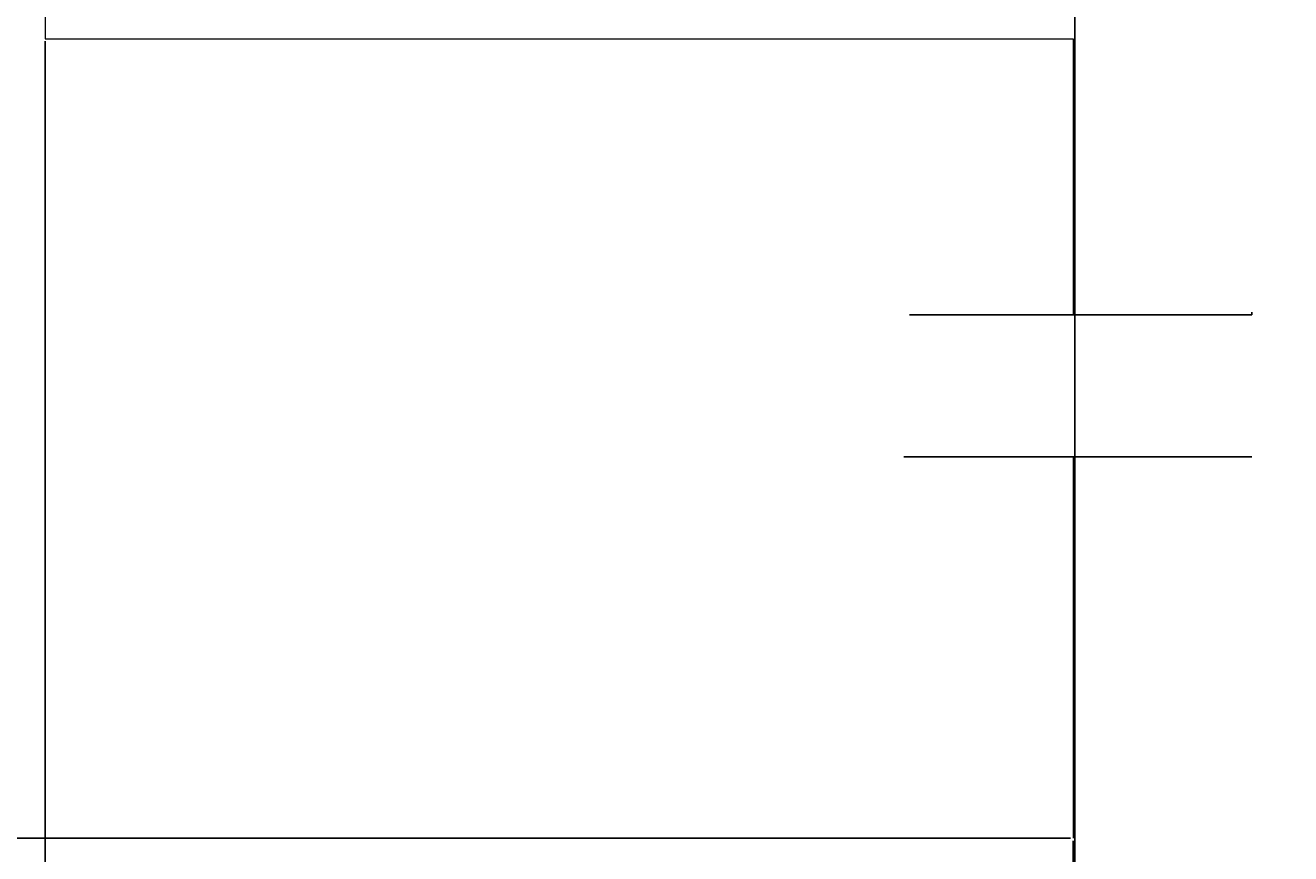
# Model space of a CAD drawing. Units: inches. Extents: x 738 to 1068, y 378 to 757.
# Tile 3 of 41: x 756 to 787, y 396 to 416. Entities that reach past the tile are written whole.
import ezdxf

# ---------------------------------------------------------------- set-up
doc = ezdxf.new("R2010")
doc.units = ezdxf.units.IN
doc.header["$MEASUREMENT"] = 0
for name, color, linetype, lineweight in [('A-ANNO-DIMS', 2, 'Continuous', 18), ('E-CTRL-CONT', 4, 'Continuous', 25), ('E-CTRL-WIRE', 7, 'Continuous', 18)]:
    doc.layers.add(name, color=color, linetype=linetype, lineweight=lineweight)
doc.styles.get("Standard").update_dxf_attribs({"font": 'arial.ttf'})
doc.dimstyles.get("Standard").update_dxf_attribs({"dimtxt": 0.18, "dimasz": 0.18, "dimexe": 0.18, "dimexo": 0.0625, "dimgap": 0.09, "dimtad": 0, "dimtih": 1, "dimtoh": 1, "dimdec": 4, "dimzin": 0, "dimdsep": 46, "dimtxsty": 'Standard', "dimcen": 0.09, "dimadec": 0, "dimazin": 0, "dimtfac": 1, "dimtdec": 4, "dimtofl": 0, "dimtmove": 0, "dimatfit": 3, "dimfxl": 1, "dimtolj": 1, "dimtzin": 0, "dimarcsym": 0})

# ---------------------------------------------------------------- blocks, each defined once
blk = doc.blocks.new('MCR-IO-CONTACT-NO')
for p, q in [((0.136, 3.468), (8.506, 3.468)), ((8.506, 3.468), (8.506, 3.536)), ((0, 0), (8.506, 0))]:
    blk.add_line(p, q)
blk = doc.blocks.new('*D17')
at = {"layer": 'A-ANNO-DIMS', "color": 0, "lineweight": -2, "transparency": 16777216}
for p, q in [((756.324, 415.842), (756.324, 378.239)), ((1050.049, 415.919), (1050.049, 378.239)), ((756.504, 378.419), (902.791, 378.419)), ((1049.869, 378.419), (903.582, 378.419))]:
    blk.add_line(p, q, dxfattribs=at)
at = {"layer": 'A-ANNO-DIMS', "color": 0, "transparency": 16777216}
for points in [[(756.504, 378.449), (756.504, 378.389), (756.324, 378.419)], [(1049.869, 378.449), (1049.869, 378.389), (1050.049, 378.419)]]:
    blk.add_solid(points, dxfattribs=at)
at = {"layer": 'Defpoints', "color": 0, "transparency": 16777216}
for p in [(1050.049, 415.982), (756.324, 415.904), (1050.049, 378.419)]:
    blk.add_point(p, dxfattribs=at)
at = {"layer": 'A-ANNO-DIMS', "color": 0, "transparency": 16777216, "insert": (903.186, 378.419), "char_height": 0.18, "attachment_point": 5}
blk.add_mtext('\\A1;293.7', dxfattribs=at)
blk = doc.blocks.new('*D19')
at = {"layer": 'A-ANNO-DIMS', "color": 0, "lineweight": -2, "transparency": 16777216}
for p, q in [((781.422, 446.265), (738.194, 446.265)), ((738.374, 446.085), (738.374, 421.499)), ((738.374, 396.549), (738.374, 421.135)), ((781.385, 396.369), (738.194, 396.369))]:
    blk.add_line(p, q, dxfattribs=at)
at = {"layer": 'A-ANNO-DIMS', "color": 0, "transparency": 16777216}
for points in [[(738.344, 446.085), (738.404, 446.085), (738.374, 446.265)], [(738.344, 396.549), (738.404, 396.549), (738.374, 396.369)]]:
    blk.add_solid(points, dxfattribs=at)
at = {"layer": 'Defpoints', "color": 0, "transparency": 16777216}
for p in [(738.374, 446.265), (781.485, 446.265), (781.447, 396.369)]:
    blk.add_point(p, dxfattribs=at)
at = {"layer": 'A-ANNO-DIMS', "color": 0, "transparency": 16777216, "insert": (738.374, 421.317), "char_height": 0.18, "attachment_point": 5}
blk.add_mtext('\\A1;49.9', dxfattribs=at)
blk = doc.blocks.new('*D25')
at = {"layer": 'A-ANNO-DIMS', "color": 0, "lineweight": -2, "transparency": 16777216}
for p, q in [((781.49, 646.923), (781.49, 378.239)), ((803.522, 646.923), (803.522, 378.239)), ((781.67, 378.419), (792.111, 378.419)), ((803.342, 378.419), (792.901, 378.419))]:
    blk.add_line(p, q, dxfattribs=at)
at = {"layer": 'A-ANNO-DIMS', "color": 0, "transparency": 16777216}
for points in [[(781.67, 378.449), (781.67, 378.389), (781.49, 378.419)], [(803.342, 378.449), (803.342, 378.389), (803.522, 378.419)]]:
    blk.add_solid(points, dxfattribs=at)
at = {"layer": 'Defpoints', "color": 0, "transparency": 16777216}
for p in [(781.49, 646.985), (803.522, 646.985), (803.522, 378.419)]:
    blk.add_point(p, dxfattribs=at)
at = {"layer": 'A-ANNO-DIMS', "color": 0, "transparency": 16777216, "insert": (792.506, 378.419), "char_height": 0.18, "attachment_point": 5}
blk.add_mtext('\\A1;22.03', dxfattribs=at)
blk = doc.blocks.new('*D34')
at = {"layer": 'A-ANNO-DIMS', "color": 0, "lineweight": -2, "transparency": 16777216}
for p, q in [((781.49, 686.266), (781.49, 378.239)), ((830.489, 686.266), (830.489, 378.239)), ((781.67, 378.419), (805.767, 378.419)), ((830.309, 378.419), (806.212, 378.419))]:
    blk.add_line(p, q, dxfattribs=at)
at = {"layer": 'A-ANNO-DIMS', "color": 0, "transparency": 16777216}
for points in [[(781.67, 378.449), (781.67, 378.389), (781.49, 378.419)], [(830.309, 378.449), (830.309, 378.389), (830.489, 378.419)]]:
    blk.add_solid(points, dxfattribs=at)
at = {"layer": 'Defpoints', "color": 0, "transparency": 16777216}
for p in [(781.49, 686.329), (830.489, 686.329), (830.489, 378.419)]:
    blk.add_point(p, dxfattribs=at)
at = {"layer": 'A-ANNO-DIMS', "color": 0, "transparency": 16777216, "insert": (805.99, 378.419), "char_height": 0.18, "attachment_point": 5}
blk.add_mtext('\\A1;49', dxfattribs=at)
blk = doc.blocks.new('*D38')
at = {"layer": 'A-ANNO-DIMS', "color": 0, "lineweight": -2, "transparency": 16777216}
for p, q in [((781.485, 593.017), (781.485, 378.239)), ((887.04, 593.067), (887.04, 378.239)), ((781.665, 378.419), (833.807, 378.419)), ((886.86, 378.419), (834.718, 378.419))]:
    blk.add_line(p, q, dxfattribs=at)
at = {"layer": 'A-ANNO-DIMS', "color": 0, "transparency": 16777216}
for points in [[(781.665, 378.449), (781.665, 378.389), (781.485, 378.419)], [(886.86, 378.449), (886.86, 378.389), (887.04, 378.419)]]:
    blk.add_solid(points, dxfattribs=at)
at = {"layer": 'Defpoints', "color": 0, "transparency": 16777216}
for p in [(781.485, 593.08), (887.04, 593.13), (887.04, 378.419)]:
    blk.add_point(p, dxfattribs=at)
at = {"layer": 'A-ANNO-DIMS', "color": 0, "transparency": 16777216, "insert": (834.263, 378.419), "char_height": 0.18, "attachment_point": 5}
blk.add_mtext('\\A1;105.56', dxfattribs=at)
blk = doc.blocks.new('*D40')
at = {"layer": 'A-ANNO-DIMS', "color": 0, "lineweight": -2, "transparency": 16777216}
for p, q in [((756.324, 415.842), (756.324, 378.239)), ((781.447, 396.307), (781.447, 378.239)), ((756.504, 378.419), (768.421, 378.419)), ((781.267, 378.419), (769.35, 378.419))]:
    blk.add_line(p, q, dxfattribs=at)
at = {"layer": 'A-ANNO-DIMS', "color": 0, "transparency": 16777216}
for points in [[(756.504, 378.449), (756.504, 378.389), (756.324, 378.419)], [(781.267, 378.449), (781.267, 378.389), (781.447, 378.419)]]:
    blk.add_solid(points, dxfattribs=at)
at = {"layer": 'Defpoints', "color": 0, "transparency": 16777216}
for p in [(756.324, 415.904), (781.447, 396.369), (781.447, 378.419)]:
    blk.add_point(p, dxfattribs=at)
at = {"layer": 'A-ANNO-DIMS', "color": 0, "transparency": 16777216, "insert": (768.885, 378.419), "char_height": 0.18, "attachment_point": 5}
blk.add_mtext('\\A1;25.124', dxfattribs=at)

msp = doc.modelspace()

# ---------------------------------------------------------------- linework, layer by layer
at = {"layer": 'E-CTRL-WIRE'}
for p, q in [((756.3236, 446.2651), (756.3236, 415.904)), ((756.3236, 415.904), (781.4474, 415.904)), ((781.4474, 415.904), (781.4474, 409.1572)), ((781.4474, 405.6894), (781.4474, 396.3691))]:
    msp.add_line(p, q, dxfattribs=at)

# ---------------------------------------------------------------- block references
at = {"layer": 'E-CTRL-CONT'}
msp.add_blockref('MCR-IO-CONTACT-NO', (777.311, 405.6894), dxfattribs=at)

# ---------------------------------------------------------------- dimensions: what is measured, and where the dimension line sits
at = {"layer": 'A-ANNO-DIMS'}
for base, p1, p2, override, picture, middle in [((830.4893, 378.4191), (781.4897, 686.329), (830.4893, 686.329), {"dimdec": 0, "dimlfac": 1, "dimrnd": 0, "dimzin": 0, "dimdsep": 46, "dimlunit": 2}, '*D34', (805.9895, 378.4191)), ((803.5218, 378.4191), (781.4897, 646.9853), (803.5218, 646.9853), {"dimdec": 2, "dimlfac": 1, "dimrnd": 0, "dimzin": 0, "dimdsep": 46, "dimlunit": 2}, '*D25', (792.5057, 378.4191)), ((887.0404, 378.4191), (781.4846, 593.0796), (887.0404, 593.1296), {"dimdec": 2, "dimlfac": 1, "dimrnd": 0, "dimzin": 0, "dimdsep": 46, "dimlunit": 2}, '*D38', (834.2625, 378.4191)), ((1050.0492, 378.4191), (756.3236, 415.904), (1050.0492, 415.982), {"dimdec": 1, "dimlfac": 1, "dimrnd": 0, "dimzin": 0, "dimdsep": 46, "dimlunit": 2}, '*D17', (903.1864, 378.4191)), ((781.4474, 378.4191), (756.3236, 415.904), (781.4474, 396.3691), {"dimdec": 3, "dimlfac": 1, "dimrnd": 0, "dimzin": 0, "dimdsep": 46, "dimlunit": 2}, '*D40', (768.8855, 378.4191))]:
    dim = msp.add_linear_dim(base=base, p1=p1, p2=p2, dimstyle='Standard', override=override, dxfattribs=at)
    dim.commit()
    dim.dimension.update_dxf_attribs({"geometry": picture, "text_midpoint": middle})
dim = msp.add_linear_dim(base=(738.3736, 446.2651), p1=(781.4474, 396.3691), p2=(781.4846, 446.2651), angle=90, dimstyle='Standard', override={"dimdec": 1, "dimlfac": 1, "dimrnd": 0, "dimzin": 0, "dimdsep": 46, "dimlunit": 2}, dxfattribs=at)
dim.commit()
dim.dimension.update_dxf_attribs({"geometry": '*D19', "text_midpoint": (738.3736, 421.3171)})

doc.saveas('drawing.dxf')
